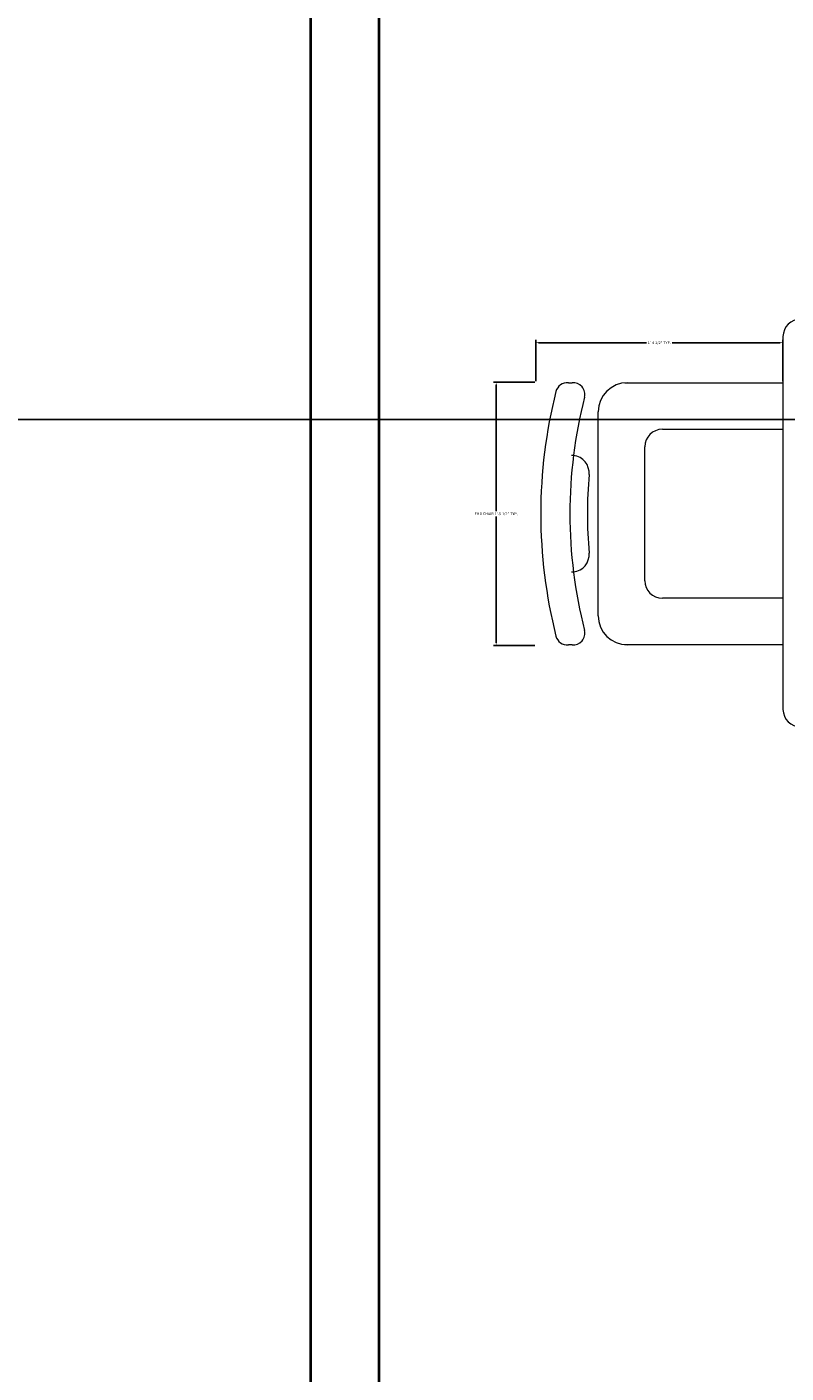
# Model space of a CAD drawing. Units: inches. Extents: x 182 to 1022, y -617 to 111.
# Tile 19 of 33: x 298 to 348, y -120 to -31. Entities that reach past the tile are written whole.
import ezdxf

# ---------------------------------------------------------------- set-up
doc = ezdxf.new("R2010")
doc.units = ezdxf.units.IN
doc.header["$MEASUREMENT"] = 0
doc.layers.add('A-ANNO-DIMS', color=2, linetype='Continuous', lineweight=18)
doc.layers.add('wall', color=1, linetype='Continuous', lineweight=40)
doc.layers.add('furniture', color=50, linetype='Continuous', lineweight=15, transparency=0.8)
doc.styles.get("Standard").update_dxf_attribs({"font": 'arial.ttf'})
doc.dimstyles.get("Standard").update_dxf_attribs({"dimtxt": 0.18, "dimasz": 0.18, "dimexe": 0.18, "dimexo": 0.0625, "dimgap": 0.09, "dimtad": 0, "dimtih": 1, "dimtoh": 1, "dimdec": 1, "dimzin": 0, "dimdsep": 46, "dimlunit": 4, "dimtxsty": 'Standard', "dimcen": 0.09, "dimadec": 0, "dimazin": 0, "dimtfac": 1, "dimtdec": 1, "dimtofl": 0, "dimtmove": 0, "dimatfit": 3, "dimfxl": 1, "dimtolj": 1, "dimtzin": 0, "dimarcsym": 0})

# ---------------------------------------------------------------- blocks, each defined once
blk = doc.blocks.new('DINING-CHAIR-END')
for p, q in [((5.528, 17.269), (5.924, 17.269)), ((5.703, 17.269), (15.947, 17.269)), ((3.784, 1.919), (3.784, 15.35)), ((8.006, 14.199), (15.947, 14.199)), ((2.157, 12.472), (2.035, 12.472)), ((6.854, 4.222), (6.854, 13.048)), ((2.157, 4.797), (2.035, 4.797)), ((15.947, 3.07), (8.006, 3.07)), ((5.924, 0), (5.528, 0)), ((15.947, 0), (5.703, 0))]:
    blk.add_line(p, q)
for centre, radius, start, end in [((1.744, 16.502), 0.768, 84.07842, 165.85295), ((1.941, 18.41), 1.151, 264.07842, 275.92158), ((2.139, 16.502), 0.768, 345.67863, 95.92158), ((5.703, 15.35), 1.919, 90, 180), ((32.955, 8.635), 32.955, 165.85295, 194.14705), ((32.955, 8.635), 31.036, 165.67863, 194.32137), ((8.006, 13.048), 1.151, 90, 180), ((2.035, 11.321), 1.151, 355.03465, 83.97191), ((32.955, 8.635), 29.885, 175.03465, 184.96535), ((2.035, 5.948), 1.151, 276.02809, 4.96535), ((8.006, 4.222), 1.151, 180, 270), ((5.703, 1.919), 1.919, 180, 270), ((2.139, 0.768), 0.768, 264.07842, 14.32137), ((1.744, 0.768), 0.768, 194.14705, 275.92158), ((1.941, -1.141), 1.151, 84.07842, 95.92158)]:
    blk.add_arc(centre, radius, start, end)
blk = doc.blocks.new('*D24')
at = {"layer": 'A-ANNO-DIMS', "color": 0, "lineweight": -2, "transparency": 16777216}
for p, q in [((331.123, -54.356), (328.405, -54.356)), ((328.585, -54.536), (328.585, -62.842)), ((328.585, -71.515), (328.585, -63.208)), ((331.123, -71.695), (328.405, -71.695))]:
    blk.add_line(p, q, dxfattribs=at)
at = {"layer": 'A-ANNO-DIMS', "color": 0, "transparency": 16777216}
for points in [[(328.555, -54.536), (328.615, -54.536), (328.585, -54.356)], [(328.555, -71.515), (328.615, -71.515), (328.585, -71.695)]]:
    blk.add_solid(points, dxfattribs=at)
at = {"layer": 'Defpoints', "color": 0, "transparency": 16777216}
for p in [(328.585, -54.356), (331.186, -54.356), (331.186, -71.695)]:
    blk.add_point(p, dxfattribs=at)
at = {"layer": 'A-ANNO-DIMS', "color": 0, "transparency": 16777216, "insert": (328.585, -63.025), "char_height": 0.18, "attachment_point": 5}
blk.add_mtext('\\A1;END CHAIR 1\'-5 1/2" TYP.', dxfattribs=at)
blk = doc.blocks.new('*D25')
at = {"layer": 'A-ANNO-DIMS', "color": 0, "lineweight": -2, "transparency": 16777216}
for p, q in [((331.186, -54.293), (331.186, -51.575)), ((331.366, -51.755), (338.486, -51.755)), ((347.286, -51.755), (340.166, -51.755)), ((347.466, -54.293), (347.466, -51.575))]:
    blk.add_line(p, q, dxfattribs=at)
at = {"layer": 'A-ANNO-DIMS', "color": 0, "transparency": 16777216}
for points in [[(331.366, -51.725), (331.366, -51.785), (331.186, -51.755)], [(347.286, -51.725), (347.286, -51.785), (347.466, -51.755)]]:
    blk.add_solid(points, dxfattribs=at)
at = {"layer": 'Defpoints', "color": 0, "transparency": 16777216}
for p in [(347.466, -51.755), (331.186, -54.356), (347.466, -54.356)]:
    blk.add_point(p, dxfattribs=at)
at = {"layer": 'A-ANNO-DIMS', "color": 0, "transparency": 16777216, "insert": (339.326, -51.755), "char_height": 0.18, "attachment_point": 5}
blk.add_mtext('\\A1;1\'-4 1/2" TYP.', dxfattribs=at)
blk = doc.blocks.new('*D43')
at = {"layer": 'A-ANNO-DIMS', "color": 0, "lineweight": -2, "transparency": 16777216}
for p, q in [((556.299, -9.373), (186.381, -9.373)), ((186.561, -9.553), (186.561, -32.91)), ((186.561, -56.633), (186.561, -33.276)), ((556.299, -56.813), (186.381, -56.813))]:
    blk.add_line(p, q, dxfattribs=at)
at = {"layer": 'A-ANNO-DIMS', "color": 0, "transparency": 16777216}
for points in [[(186.531, -9.553), (186.591, -9.553), (186.561, -9.373)], [(186.531, -56.633), (186.591, -56.633), (186.561, -56.813)]]:
    blk.add_solid(points, dxfattribs=at)
at = {"layer": 'Defpoints', "color": 0, "transparency": 16777216}
for p in [(556.361, -9.373), (186.561, -56.813), (556.361, -56.813)]:
    blk.add_point(p, dxfattribs=at)
at = {"layer": 'A-ANNO-DIMS', "color": 0, "transparency": 16777216, "insert": (186.561, -33.093), "char_height": 0.18, "attachment_point": 5}
blk.add_mtext('\\A1;3\'-11 1/2"', dxfattribs=at)

msp = doc.modelspace()

# ---------------------------------------------------------------- linework, layer by layer
at = {"layer": 'furniture'}
msp.add_line((347.466, -51.351), (347.466, -75.911), dxfattribs=at)
for centre, start, end in [((348.618, -51.351), 90, 180), ((348.618, -75.911), 180, 270)]:
    msp.add_arc(centre, 1.151, start, end, dxfattribs=at)
at = {"layer": 'wall'}
for p, q in [((316.361, -9.373), (316.361, -121.873)), ((320.861, -9.373), (320.861, -121.873))]:
    msp.add_line(p, q, dxfattribs=at)

# ---------------------------------------------------------------- block references
at = {"layer": 'furniture'}
msp.add_blockref('DINING-CHAIR-END', (331.519, -71.66), dxfattribs=at)

# ---------------------------------------------------------------- dimensions: what is measured, and where the dimension line sits
at = {"layer": 'A-ANNO-DIMS'}
dim = msp.add_linear_dim(base=(186.561, -56.813), p1=(556.361, -9.373), p2=(556.361, -56.813), angle=90, dimstyle='Standard', override={"dimdec": 1, "dimlfac": 1, "dimrnd": 0, "dimzin": 1, "dimdsep": 46, "dimlunit": 4, "dimfrac": 2}, dxfattribs=at)
dim.commit()
dim.dimension.update_dxf_attribs({"geometry": '*D43', "text_midpoint": (186.561, -33.093)})
dim = msp.add_linear_dim(base=(347.466, -51.755), p1=(331.186, -54.356), p2=(347.466, -54.356), text='<> TYP.', dimstyle='Standard', override={"dimdec": 1, "dimlfac": 1, "dimrnd": 0, "dimzin": 1, "dimdsep": 46, "dimlunit": 4, "dimfrac": 2}, dxfattribs=at)
dim.commit()
dim.dimension.update_dxf_attribs({"geometry": '*D25', "text_midpoint": (339.326, -51.755)})
dim = msp.add_linear_dim(base=(328.585, -54.356), p1=(331.186, -71.695), p2=(331.186, -54.356), angle=90, text='END CHAIR <> TYP.', dimstyle='Standard', override={"dimdec": 1, "dimlfac": 1, "dimrnd": 0, "dimzin": 1, "dimdsep": 46, "dimlunit": 4, "dimfrac": 2}, dxfattribs=at)
dim.commit()
dim.dimension.update_dxf_attribs({"geometry": '*D24', "text_midpoint": (328.585, -63.025)})

doc.saveas('drawing.dxf')
